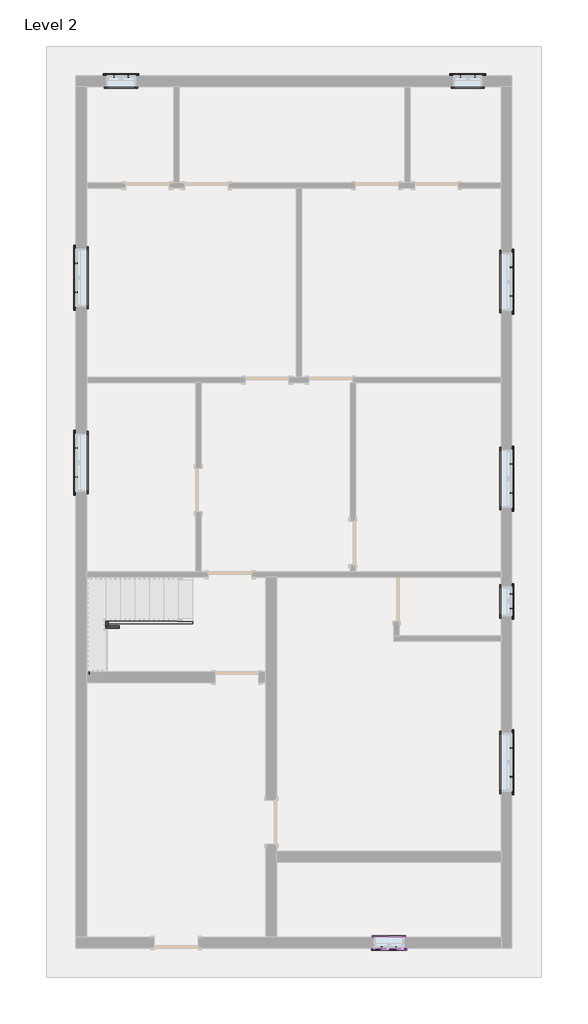
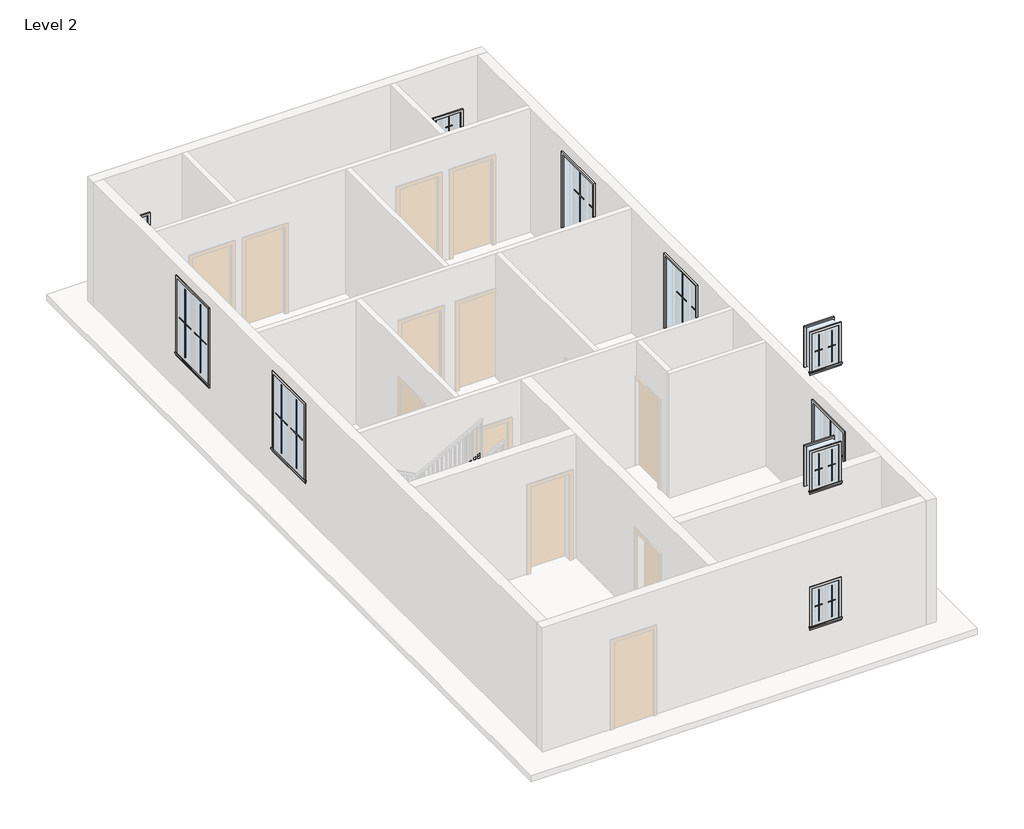
# One storey, part 3 of 3: 44 proxies, 6 members.
"""IFC4 building model written with IfcOpenShell, lengths in millimetres."""

from ifc_helpers import new_model, si_unit, frame, origin, place, context, project, spatial, polyline, outline, extrude, transform, mapped, element, save
from components import muntin_pattern_2x2_muntin_pattern_2x2_2b4d9f72, muntin_pattern_2x2_muntin_pattern_2x2_ef995ed3, muntin_pattern_2x2_muntin_pattern_2x2_53152e2c, muntin_pattern_2x2_muntin_pattern_2x2_e8f3e573, trim_window_exterior_flat_with_sill_b7e4d11c, trim_window_exterior_flat_with_sill_a665a915, trim_window_interior_flat_picture_frame_936b8d2a, trim_window_interior_flat_picture_frame_d485c387

model = new_model("IFC4")

# Units and contexts
model_context = context("Model", 3, world=origin())
ifc_project = project(units=[si_unit("LENGTHUNIT", "METRE", prefix="MILLI")], contexts=[model_context])

# Site, building, storey
site = spatial("IfcSite", under=ifc_project)
building = spatial("IfcBuilding", under=site)
storey = spatial("IfcBuildingStorey", under=building, Name="Level 2", Elevation=3048.0)

# Proxies
placement = place(None, origin())
muntin_pattern_2x2_muntin_pattern_2x2_shape = muntin_pattern_2x2_muntin_pattern_2x2_2b4d9f72(model_context)
element("IfcBuildingElementProxy", 1, Name="Muntin Pattern_2x2 : Muntin Pattern_2x2", ObjectType="Muntin Pattern_2x2 : Muntin Pattern_2x2", at=placement, inside=storey, context=model_context, shape_type="MappedRepresentation", body=[
    mapped(muntin_pattern_2x2_muntin_pattern_2x2_shape, transform((1279.525, 5811.8375, 4032.25), x_axis=(0.0, 1.0, 0.0), y_axis=(-1.0, 0.0, 0.0), z_axis=(0.0, 0.0, 1.0))),
])
element("IfcBuildingElementProxy", 2, Name="Muntin Pattern_2x2 : Muntin Pattern_2x2", ObjectType="Muntin Pattern_2x2 : Muntin Pattern_2x2", at=placement, inside=storey, context=model_context, shape_type="MappedRepresentation", body=[
    mapped(muntin_pattern_2x2_muntin_pattern_2x2_shape, transform((1279.525, 9685.3375, 4032.25), x_axis=(0.0, 1.0, 0.0), y_axis=(-1.0, 0.0, 0.0), z_axis=(0.0, 0.0, 1.0))),
])
element("IfcBuildingElementProxy", 3, Name="Muntin Pattern_2x2 : Muntin Pattern_2x2", ObjectType="Muntin Pattern_2x2 : Muntin Pattern_2x2", at=placement, inside=storey, context=model_context, shape_type="MappedRepresentation", body=[
    mapped(muntin_pattern_2x2_muntin_pattern_2x2_shape, transform((10404.475, 10209.2125, 4032.25), x_axis=(0.0, -1.0, 0.0), y_axis=(1.0, 0.0, 0.0), z_axis=(0.0, 0.0, 1.0))),
])
element("IfcBuildingElementProxy", 4, Name="Muntin Pattern_2x2 : Muntin Pattern_2x2", ObjectType="Muntin Pattern_2x2 : Muntin Pattern_2x2", at=placement, inside=storey, context=model_context, shape_type="MappedRepresentation", body=[
    mapped(muntin_pattern_2x2_muntin_pattern_2x2_shape, transform((10404.475, 6081.7125, 4032.25), x_axis=(0.0, -1.0, 0.0), y_axis=(1.0, 0.0, 0.0), z_axis=(0.0, 0.0, 1.0))),
])
element("IfcBuildingElementProxy", 5, Name="Muntin Pattern_2x2 : Muntin Pattern_2x2", ObjectType="Muntin Pattern_2x2 : Muntin Pattern_2x2", at=placement, inside=storey, context=model_context, shape_type="MappedRepresentation", body=[
    mapped(muntin_pattern_2x2_muntin_pattern_2x2_shape, transform((10404.475, 138.1125, 4032.25), x_axis=(0.0, -1.0, 0.0), y_axis=(1.0, 0.0, 0.0), z_axis=(0.0, 0.0, 1.0))),
])
muntin_pattern_2x2_muntin_pattern_2x2_2_shape = muntin_pattern_2x2_muntin_pattern_2x2_ef995ed3(model_context)
element("IfcBuildingElementProxy", 6, Name="Muntin Pattern_2x2 : Muntin Pattern_2x2", ObjectType="Muntin Pattern_2x2 : Muntin Pattern_2x2", at=placement, inside=storey, context=model_context, shape_type="MappedRepresentation", body=[
    mapped(muntin_pattern_2x2_muntin_pattern_2x2_2_shape, transform((1279.525, 6418.2625, 4032.25), x_axis=(0.0, -1.0, 0.0), y_axis=(1.0, 0.0, 0.0), z_axis=(0.0, 0.0, 1.0))),
])
element("IfcBuildingElementProxy", 7, Name="Muntin Pattern_2x2 : Muntin Pattern_2x2", ObjectType="Muntin Pattern_2x2 : Muntin Pattern_2x2", at=placement, inside=storey, context=model_context, shape_type="MappedRepresentation", body=[
    mapped(muntin_pattern_2x2_muntin_pattern_2x2_2_shape, transform((1279.525, 10291.7625, 4032.25), x_axis=(0.0, -1.0, 0.0), y_axis=(1.0, 0.0, 0.0), z_axis=(0.0, 0.0, 1.0))),
])
element("IfcBuildingElementProxy", 8, Name="Muntin Pattern_2x2 : Muntin Pattern_2x2", ObjectType="Muntin Pattern_2x2 : Muntin Pattern_2x2", at=placement, inside=storey, context=model_context, shape_type="MappedRepresentation", body=[
    mapped(muntin_pattern_2x2_muntin_pattern_2x2_2_shape, transform((10404.475, 9602.7875, 4032.25), x_axis=(0.0, 1.0, 0.0), y_axis=(-1.0, 0.0, 0.0), z_axis=(0.0, 0.0, 1.0))),
])
element("IfcBuildingElementProxy", 9, Name="Muntin Pattern_2x2 : Muntin Pattern_2x2", ObjectType="Muntin Pattern_2x2 : Muntin Pattern_2x2", at=placement, inside=storey, context=model_context, shape_type="MappedRepresentation", body=[
    mapped(muntin_pattern_2x2_muntin_pattern_2x2_2_shape, transform((10404.475, 5475.2875, 4032.25), x_axis=(0.0, 1.0, 0.0), y_axis=(-1.0, 0.0, 0.0), z_axis=(0.0, 0.0, 1.0))),
])
element("IfcBuildingElementProxy", 10, Name="Muntin Pattern_2x2 : Muntin Pattern_2x2", ObjectType="Muntin Pattern_2x2 : Muntin Pattern_2x2", at=placement, inside=storey, context=model_context, shape_type="MappedRepresentation", body=[
    mapped(muntin_pattern_2x2_muntin_pattern_2x2_2_shape, transform((10404.475, -468.3125, 4032.25), x_axis=(0.0, 1.0, 0.0), y_axis=(-1.0, 0.0, 0.0), z_axis=(0.0, 0.0, 1.0))),
])
muntin_pattern_2x2_muntin_pattern_2x2_3_shape = muntin_pattern_2x2_muntin_pattern_2x2_53152e2c(model_context)
element("IfcBuildingElementProxy", 11, Name="Muntin Pattern_2x2 : Muntin Pattern_2x2", ObjectType="Muntin Pattern_2x2 : Muntin Pattern_2x2", at=placement, inside=storey, context=model_context, shape_type="MappedRepresentation", body=[
    mapped(muntin_pattern_2x2_muntin_pattern_2x2_3_shape, transform((10404.475, 3357.5625, 4032.25), x_axis=(0.0, -1.0, 0.0), y_axis=(1.0, 0.0, 0.0), z_axis=(0.0, 0.0, 1.0))),
])
element("IfcBuildingElementProxy", 12, Name="Muntin Pattern_2x2 : Muntin Pattern_2x2", ObjectType="Muntin Pattern_2x2 : Muntin Pattern_2x2", at=placement, inside=storey, context=model_context, shape_type="MappedRepresentation", body=[
    mapped(muntin_pattern_2x2_muntin_pattern_2x2_3_shape, transform((9336.0875, 14214.475, 4032.25), x_axis=(1.0, 0.0, 0.0), y_axis=(0.0, 1.0, 0.0), z_axis=(0.0, 0.0, 1.0))),
])
element("IfcBuildingElementProxy", 13, Name="Muntin Pattern_2x2 : Muntin Pattern_2x2", ObjectType="Muntin Pattern_2x2 : Muntin Pattern_2x2", at=placement, inside=storey, context=model_context, shape_type="MappedRepresentation", body=[
    mapped(muntin_pattern_2x2_muntin_pattern_2x2_3_shape, transform((2071.6875, 14214.475, 4032.25), x_axis=(1.0, 0.0, 0.0), y_axis=(0.0, 1.0, 0.0), z_axis=(0.0, 0.0, 1.0))),
])
element("IfcBuildingElementProxy", 14, Name="Muntin Pattern_2x2 : Muntin Pattern_2x2", ObjectType="Muntin Pattern_2x2 : Muntin Pattern_2x2", at=placement, inside=storey, context=model_context, shape_type="MappedRepresentation", body=[
    mapped(muntin_pattern_2x2_muntin_pattern_2x2_3_shape, transform((7986.7125, -4054.475, 4032.25), x_axis=(-1.0, 0.0, 0.0), y_axis=(0.0, -1.0, 0.0), z_axis=(0.0, 0.0, 1.0))),
])
element("IfcBuildingElementProxy", 15, Name="Muntin Pattern_2x2 : Muntin Pattern_2x2", ObjectType="Muntin Pattern_2x2 : Muntin Pattern_2x2", at=placement, inside=storey, context=model_context, shape_type="MappedRepresentation", body=[
    mapped(muntin_pattern_2x2_muntin_pattern_2x2_3_shape, transform((7986.7125, -4054.475, 7370.6757161), x_axis=(-1.0, 0.0, 0.0), y_axis=(0.0, -1.0, 0.0), z_axis=(0.0, 0.0, 1.0))),
])
element("IfcBuildingElementProxy", 16, Name="Muntin Pattern_2x2 : Muntin Pattern_2x2", ObjectType="Muntin Pattern_2x2 : Muntin Pattern_2x2", at=placement, inside=storey, context=model_context, shape_type="MappedRepresentation", body=[
    mapped(muntin_pattern_2x2_muntin_pattern_2x2_3_shape, transform((7986.7125, -4054.475, 10294.9373604), x_axis=(-1.0, 0.0, 0.0), y_axis=(0.0, -1.0, 0.0), z_axis=(0.0, 0.0, 1.0))),
])
muntin_pattern_2x2_muntin_pattern_2x2_4_shape = muntin_pattern_2x2_muntin_pattern_2x2_e8f3e573(model_context)
element("IfcBuildingElementProxy", 17, Name="Muntin Pattern_2x2 : Muntin Pattern_2x2", ObjectType="Muntin Pattern_2x2 : Muntin Pattern_2x2", at=placement, inside=storey, context=model_context, shape_type="MappedRepresentation", body=[
    mapped(muntin_pattern_2x2_muntin_pattern_2x2_4_shape, transform((10404.475, 3055.9375, 4032.25), x_axis=(0.0, 1.0, 0.0), y_axis=(-1.0, 0.0, 0.0), z_axis=(0.0, 0.0, 1.0))),
])
element("IfcBuildingElementProxy", 18, Name="Muntin Pattern_2x2 : Muntin Pattern_2x2", ObjectType="Muntin Pattern_2x2 : Muntin Pattern_2x2", at=placement, inside=storey, context=model_context, shape_type="MappedRepresentation", body=[
    mapped(muntin_pattern_2x2_muntin_pattern_2x2_4_shape, transform((9637.7125, 14214.475, 4032.25), x_axis=(-1.0, 0.0, 0.0), y_axis=(0.0, -1.0, 0.0), z_axis=(0.0, 0.0, 1.0))),
])
element("IfcBuildingElementProxy", 19, Name="Muntin Pattern_2x2 : Muntin Pattern_2x2", ObjectType="Muntin Pattern_2x2 : Muntin Pattern_2x2", at=placement, inside=storey, context=model_context, shape_type="MappedRepresentation", body=[
    mapped(muntin_pattern_2x2_muntin_pattern_2x2_4_shape, transform((2373.3125, 14214.475, 4032.25), x_axis=(-1.0, 0.0, 0.0), y_axis=(0.0, -1.0, 0.0), z_axis=(0.0, 0.0, 1.0))),
])
element("IfcBuildingElementProxy", 20, Name="Muntin Pattern_2x2 : Muntin Pattern_2x2", ObjectType="Muntin Pattern_2x2 : Muntin Pattern_2x2", at=placement, inside=storey, context=model_context, shape_type="MappedRepresentation", body=[
    mapped(muntin_pattern_2x2_muntin_pattern_2x2_4_shape, transform((7685.0875, -4054.475, 4032.25), x_axis=(1.0, 0.0, 0.0), y_axis=(0.0, 1.0, 0.0), z_axis=(0.0, 0.0, 1.0))),
])
element("IfcBuildingElementProxy", 21, Name="Muntin Pattern_2x2 : Muntin Pattern_2x2", ObjectType="Muntin Pattern_2x2 : Muntin Pattern_2x2", at=placement, inside=storey, context=model_context, shape_type="MappedRepresentation", body=[
    mapped(muntin_pattern_2x2_muntin_pattern_2x2_4_shape, transform((7685.0875, -4054.475, 7370.6757161), x_axis=(1.0, 0.0, 0.0), y_axis=(0.0, 1.0, 0.0), z_axis=(0.0, 0.0, 1.0))),
])
element("IfcBuildingElementProxy", 22, Name="Muntin Pattern_2x2 : Muntin Pattern_2x2", ObjectType="Muntin Pattern_2x2 : Muntin Pattern_2x2", at=placement, inside=storey, context=model_context, shape_type="MappedRepresentation", body=[
    mapped(muntin_pattern_2x2_muntin_pattern_2x2_4_shape, transform((7685.0875, -4054.475, 10294.9373604), x_axis=(1.0, 0.0, 0.0), y_axis=(0.0, 1.0, 0.0), z_axis=(0.0, 0.0, 1.0))),
])
trim_window_exterior_flat_with_sill_shape = trim_window_exterior_flat_with_sill_b7e4d11c(model_context)
element("IfcBuildingElementProxy", 23, Name="Trim-Window-Exterior-Flat : with Sill", ObjectType="Trim-Window-Exterior-Flat : with Sill", at=placement, inside=storey, context=model_context, shape_type="MappedRepresentation", body=[
    mapped(trim_window_exterior_flat_with_sill_shape, transform((1270.0, 6115.05, 5791.2), x_axis=(0.0, -1.0, 0.0), y_axis=(0.0, 0.0, 1.0), z_axis=(-1.0, 0.0, 0.0))),
])
element("IfcBuildingElementProxy", 24, Name="Trim-Window-Exterior-Flat : with Sill", ObjectType="Trim-Window-Exterior-Flat : with Sill", at=placement, inside=storey, context=model_context, shape_type="MappedRepresentation", body=[
    mapped(trim_window_exterior_flat_with_sill_shape, transform((1270.0, 9988.55, 5791.2), x_axis=(0.0, -1.0, 0.0), y_axis=(0.0, 0.0, 1.0), z_axis=(-1.0, 0.0, 0.0))),
])
element("IfcBuildingElementProxy", 25, Name="Trim-Window-Exterior-Flat : with Sill", ObjectType="Trim-Window-Exterior-Flat : with Sill", at=placement, inside=storey, context=model_context, shape_type="MappedRepresentation", body=[
    mapped(trim_window_exterior_flat_with_sill_shape, transform((10414.0, 9906.0, 5791.2), x_axis=(0.0, 1.0, 0.0), y_axis=(0.0, 0.0, 1.0), z_axis=(1.0, 0.0, 0.0))),
])
element("IfcBuildingElementProxy", 26, Name="Trim-Window-Exterior-Flat : with Sill", ObjectType="Trim-Window-Exterior-Flat : with Sill", at=placement, inside=storey, context=model_context, shape_type="MappedRepresentation", body=[
    mapped(trim_window_exterior_flat_with_sill_shape, transform((10414.0, 5778.5, 5791.2), x_axis=(0.0, 1.0, 0.0), y_axis=(0.0, 0.0, 1.0), z_axis=(1.0, 0.0, 0.0))),
])
element("IfcBuildingElementProxy", 27, Name="Trim-Window-Exterior-Flat : with Sill", ObjectType="Trim-Window-Exterior-Flat : with Sill", at=placement, inside=storey, context=model_context, shape_type="MappedRepresentation", body=[
    mapped(trim_window_exterior_flat_with_sill_shape, transform((10414.0, -165.1, 5791.2), x_axis=(0.0, 1.0, 0.0), y_axis=(0.0, 0.0, 1.0), z_axis=(1.0, 0.0, 0.0))),
])
trim_window_exterior_flat_with_sill_2_shape = trim_window_exterior_flat_with_sill_a665a915(model_context)
element("IfcBuildingElementProxy", 28, Name="Trim-Window-Exterior-Flat : with Sill", ObjectType="Trim-Window-Exterior-Flat : with Sill", at=placement, inside=storey, context=model_context, shape_type="MappedRepresentation", body=[
    mapped(trim_window_exterior_flat_with_sill_2_shape, transform((10414.0, 3206.75, 4876.8), x_axis=(0.0, 1.0, 0.0), y_axis=(0.0, 0.0, 1.0), z_axis=(1.0, 0.0, 0.0))),
])
element("IfcBuildingElementProxy", 29, Name="Trim-Window-Exterior-Flat : with Sill", ObjectType="Trim-Window-Exterior-Flat : with Sill", at=placement, inside=storey, context=model_context, shape_type="MappedRepresentation", body=[
    mapped(trim_window_exterior_flat_with_sill_2_shape, transform((9486.9, 14224.0, 4876.8), x_axis=(-1.0, 0.0, 0.0), y_axis=(0.0, 0.0, 1.0), z_axis=(0.0, 1.0, 0.0))),
])
element("IfcBuildingElementProxy", 30, Name="Trim-Window-Exterior-Flat : with Sill", ObjectType="Trim-Window-Exterior-Flat : with Sill", at=placement, inside=storey, context=model_context, shape_type="MappedRepresentation", body=[
    mapped(trim_window_exterior_flat_with_sill_2_shape, transform((2222.5, 14224.0, 4876.8), x_axis=(-1.0, 0.0, 0.0), y_axis=(0.0, 0.0, 1.0), z_axis=(0.0, 1.0, 0.0))),
])
element("IfcBuildingElementProxy", 31, Name="Trim-Window-Exterior-Flat : with Sill", ObjectType="Trim-Window-Exterior-Flat : with Sill", at=placement, inside=storey, context=model_context, shape_type="MappedRepresentation", body=[
    mapped(trim_window_exterior_flat_with_sill_2_shape, transform((7835.9, -4064.0, 4876.8), x_axis=(1.0, 0.0, 0.0), y_axis=(0.0, 0.0, 1.0), z_axis=(0.0, -1.0, 0.0))),
])
element("IfcBuildingElementProxy", 32, Name="Trim-Window-Exterior-Flat : with Sill", ObjectType="Trim-Window-Exterior-Flat : with Sill", at=placement, inside=storey, context=model_context, shape_type="MappedRepresentation", body=[
    mapped(trim_window_exterior_flat_with_sill_2_shape, transform((7835.9, -4064.0, 8215.2257161), x_axis=(1.0, 0.0, 0.0), y_axis=(0.0, 0.0, 1.0), z_axis=(0.0, -1.0, 0.0))),
])
element("IfcBuildingElementProxy", 33, Name="Trim-Window-Exterior-Flat : with Sill", ObjectType="Trim-Window-Exterior-Flat : with Sill", at=placement, inside=storey, context=model_context, shape_type="MappedRepresentation", body=[
    mapped(trim_window_exterior_flat_with_sill_2_shape, transform((7835.9, -4064.0, 11139.4873604), x_axis=(1.0, 0.0, 0.0), y_axis=(0.0, 0.0, 1.0), z_axis=(0.0, -1.0, 0.0))),
])
trim_window_interior_flat_picture_frame_shape = trim_window_interior_flat_picture_frame_936b8d2a(model_context)
element("IfcBuildingElementProxy", 34, Name="Trim-Window-Interior-Flat : Picture Frame", ObjectType="Trim-Window-Interior-Flat : Picture Frame", at=placement, inside=storey, context=model_context, shape_type="MappedRepresentation", body=[
    mapped(trim_window_interior_flat_picture_frame_shape, transform((1498.6, 6115.05, 5791.2), x_axis=(0.0, 1.0, 0.0), y_axis=(0.0, 0.0, 1.0), z_axis=(1.0, 0.0, 0.0))),
])
element("IfcBuildingElementProxy", 35, Name="Trim-Window-Interior-Flat : Picture Frame", ObjectType="Trim-Window-Interior-Flat : Picture Frame", at=placement, inside=storey, context=model_context, shape_type="MappedRepresentation", body=[
    mapped(trim_window_interior_flat_picture_frame_shape, transform((1498.6, 9988.55, 5791.2), x_axis=(0.0, 1.0, 0.0), y_axis=(0.0, 0.0, 1.0), z_axis=(1.0, 0.0, 0.0))),
])
element("IfcBuildingElementProxy", 36, Name="Trim-Window-Interior-Flat : Picture Frame", ObjectType="Trim-Window-Interior-Flat : Picture Frame", at=placement, inside=storey, context=model_context, shape_type="MappedRepresentation", body=[
    mapped(trim_window_interior_flat_picture_frame_shape, transform((10185.4, 9906.0, 5791.2), x_axis=(0.0, -1.0, 0.0), y_axis=(0.0, 0.0, 1.0), z_axis=(-1.0, 0.0, 0.0))),
])
element("IfcBuildingElementProxy", 37, Name="Trim-Window-Interior-Flat : Picture Frame", ObjectType="Trim-Window-Interior-Flat : Picture Frame", at=placement, inside=storey, context=model_context, shape_type="MappedRepresentation", body=[
    mapped(trim_window_interior_flat_picture_frame_shape, transform((10185.4, 5778.5, 5791.2), x_axis=(0.0, -1.0, 0.0), y_axis=(0.0, 0.0, 1.0), z_axis=(-1.0, 0.0, 0.0))),
])
element("IfcBuildingElementProxy", 38, Name="Trim-Window-Interior-Flat : Picture Frame", ObjectType="Trim-Window-Interior-Flat : Picture Frame", at=placement, inside=storey, context=model_context, shape_type="MappedRepresentation", body=[
    mapped(trim_window_interior_flat_picture_frame_shape, transform((10185.4, -165.1, 5791.2), x_axis=(0.0, -1.0, 0.0), y_axis=(0.0, 0.0, 1.0), z_axis=(-1.0, 0.0, 0.0))),
])
trim_window_interior_flat_picture_frame_2_shape = trim_window_interior_flat_picture_frame_d485c387(model_context)
element("IfcBuildingElementProxy", 39, Name="Trim-Window-Interior-Flat : Picture Frame", ObjectType="Trim-Window-Interior-Flat : Picture Frame", at=placement, inside=storey, context=model_context, shape_type="MappedRepresentation", body=[
    mapped(trim_window_interior_flat_picture_frame_2_shape, transform((10185.4, 3206.75, 4876.8), x_axis=(0.0, -1.0, 0.0), y_axis=(0.0, 0.0, 1.0), z_axis=(-1.0, 0.0, 0.0))),
])
element("IfcBuildingElementProxy", 40, Name="Trim-Window-Interior-Flat : Picture Frame", ObjectType="Trim-Window-Interior-Flat : Picture Frame", at=placement, inside=storey, context=model_context, shape_type="MappedRepresentation", body=[
    mapped(trim_window_interior_flat_picture_frame_2_shape, transform((9486.9, 13995.4, 4876.8), x_axis=(1.0, 0.0, 0.0), y_axis=(0.0, 0.0, 1.0), z_axis=(0.0, -1.0, 0.0))),
])
element("IfcBuildingElementProxy", 41, Name="Trim-Window-Interior-Flat : Picture Frame", ObjectType="Trim-Window-Interior-Flat : Picture Frame", at=placement, inside=storey, context=model_context, shape_type="MappedRepresentation", body=[
    mapped(trim_window_interior_flat_picture_frame_2_shape, transform((2222.5, 13995.4, 4876.8), x_axis=(1.0, 0.0, 0.0), y_axis=(0.0, 0.0, 1.0), z_axis=(0.0, -1.0, 0.0))),
])
element("IfcBuildingElementProxy", 42, Name="Trim-Window-Interior-Flat : Picture Frame", ObjectType="Trim-Window-Interior-Flat : Picture Frame", at=placement, inside=storey, context=model_context, shape_type="MappedRepresentation", body=[
    mapped(trim_window_interior_flat_picture_frame_2_shape, transform((7835.9, -3835.4, 4876.8), x_axis=(-1.0, 0.0, 0.0), y_axis=(0.0, 0.0, 1.0), z_axis=(0.0, 1.0, 0.0))),
])
element("IfcBuildingElementProxy", 43, Name="Trim-Window-Interior-Flat : Picture Frame", ObjectType="Trim-Window-Interior-Flat : Picture Frame", at=placement, inside=storey, context=model_context, shape_type="MappedRepresentation", body=[
    mapped(trim_window_interior_flat_picture_frame_2_shape, transform((7835.9, -3835.4, 8215.2257161), x_axis=(-1.0, 0.0, 0.0), y_axis=(0.0, 0.0, 1.0), z_axis=(0.0, 1.0, 0.0))),
])
element("IfcBuildingElementProxy", 44, Name="Trim-Window-Interior-Flat : Picture Frame", ObjectType="Trim-Window-Interior-Flat : Picture Frame", at=placement, inside=storey, context=model_context, shape_type="MappedRepresentation", body=[
    mapped(trim_window_interior_flat_picture_frame_2_shape, transform((7835.9, -3835.4, 11139.4873604), x_axis=(-1.0, 0.0, 0.0), y_axis=(0.0, 0.0, 1.0), z_axis=(0.0, 1.0, 0.0))),
])

# Members
element("IfcMember", 45, ObjectType="Stringer - 2\" Width", at=placement, inside=storey, context=model_context, shape_type="SweptSolid", body=[
    extrude(outline(polyline([(3048.0, 3727.9146873), (3255.5983948, 3727.9146873), (4243.3761726, 1949.9146873), (3894.6974984, 1949.9146873), (3048.0, 3473.9701845), (3048.0, 3727.9146873)])), frame((0.0, 2743.2, 0.0), z_axis=(0.0, 1.0, 0.0), x_axis=(0.0, 0.0, 1.0)), (0.0, 0.0, 1.0), 50.8),
])
element("IfcMember", 46, ObjectType="Stringer - 2\" Width", at=placement, inside=storey, context=model_context, shape_type="SweptSolid", body=[
    extrude(outline(polyline([(1899.1146873, 2794.0), (1949.9146873, 2794.0), (1949.9146873, 2692.4), (1899.1146873, 2692.4), (1899.1146873, 2794.0)])), frame((0.0, 0.0, 4004.7333333), z_axis=(0.0, 0.0, 1.0), x_axis=(1.0, 0.0, 0.0)), (0.0, 0.0, 1.0), 304.8),
])
element("IfcMember", 47, ObjectType="Stringer - 2\" Width", at=placement, inside=storey, context=model_context, shape_type="SweptSolid", body=[
    extrude(outline(polyline([(4440.9317281, 1899.1146873), (4092.253054, 1899.1146873), (5108.253054, 3727.9146873), (5456.9317281, 3727.9146873), (4440.9317281, 1899.1146873)])), frame((0.0, 2641.6, 0.0), z_axis=(0.0, 1.0, 0.0), x_axis=(0.0, 0.0, 1.0)), (0.0, 0.0, 1.0), 50.8),
])
element("IfcMember", 48, ObjectType="Stringer - 2\" Width", at=placement, inside=storey, context=model_context, shape_type="SweptSolid", body=[
    extrude(outline(polyline([(3048.0, 3727.9146873), (3255.5983948, 3727.9146873), (4309.5333333, 1830.8317979), (4309.5333333, 1498.6), (4145.4278803, 1498.6), (3048.0, 3473.9701845), (3048.0, 3727.9146873)])), frame((0.0, 3708.4, 0.0), z_axis=(0.0, 1.0, 0.0), x_axis=(0.0, 0.0, 1.0)), (0.0, 0.0, 1.0), 50.8),
])
element("IfcMember", 49, ObjectType="Stringer - 2\" Width", at=placement, inside=storey, context=model_context, shape_type="SweptSolid", body=[
    extrude(outline(polyline([(1447.8, 3759.2), (1498.6, 3759.2), (1498.6, 1727.2), (1447.8, 1727.2), (1447.8, 3759.2)])), frame((0.0, 0.0, 4004.7333333), z_axis=(0.0, 0.0, 1.0), x_axis=(1.0, 0.0, 0.0)), (0.0, 0.0, 1.0), 304.8),
])
element("IfcMember", 50, ObjectType="Stringer - 2\" Width", at=placement, inside=storey, context=model_context, shape_type="SweptSolid", body=[
    extrude(outline(polyline([(4190.2013463, 1447.8), (4004.7333333, 1447.8), (4004.7333333, 1741.5791901), (5108.253054, 3727.9146873), (5456.9317281, 3727.9146873), (4190.2013463, 1447.8)])), frame((0.0, 1676.4, 0.0), z_axis=(0.0, 1.0, 0.0), x_axis=(0.0, 0.0, 1.0)), (0.0, 0.0, 1.0), 50.8),
])

save(model, "model.ifc")

# Revit data of these elements
# Type "Muntin Pattern_2x2 : Muntin Pattern_2x2"
#   Width [instance default] = 4' - 0"
#   Thickness = 0' - 0 1/2"
#   Height [instance default] = 4' - 0"
#   Distance = 0' - 0 3/4"
#   Interior Material [instance default] = none
#   Exterior Material [instance default] = none
#   Default Elevation = 0
# Type "Trim-Window-Exterior-Flat : with Sill"
#   Trim Width = 0' - 2 1/4"
#   Trim Thickness_Picture Frame = 0' - 1 1/4"
#   Trim Thickness_with Sill = 0' - 0 3/4"
#   Sill Thickness = 0' - 1 1/4"
#   Opening Width [instance default] = 2' - 0"
#   Opening Height [instance default] = 3' - 0"
#   Default Elevation = 4' - 0"
#   Sill = yes
#   Picture Frame = no
#   Trim Material [instance default] = none
# Type "Trim-Window-Interior-Flat : Picture Frame"
#   Trim Thickness_Picture Frame = 0' - 1 1/4"
#   Trim Width = 0' - 2 1/4"
#   Trim Thickness_with Sill = 0' - 0 3/4"
#   Sill Thickness = 0' - 1 1/4"
#   Opening Width [instance default] = 2' - 0"
#   Opening Height [instance default] = 3' - 0"
#   Default Elevation = 4' - 0"
#   Sill = no
#   Picture Frame = yes
#   Trim Material [instance default] = none
# Elements 1, 2, 3, 4, 5, 6, 7, 8, 9, 10 (IfcBuildingElementProxy, "Muntin Pattern_2x2 : Muntin Pattern_2x2")
#   Width = 1' - 6 5/8"
#   Height = 5' - 6 1/2"
#   Interior Material = Wood - Stained
#   Exterior Material = Clad - White
#   Phase Created = New Construction
#   Materials on its faces: "Clad - White", "Wood - Stained"
# Elements 11, 12, 13, 14, 15, 16, 17, 18, 19, 20, 21, 22 (IfcBuildingElementProxy, "Muntin Pattern_2x2 : Muntin Pattern_2x2")
#   Width = 0' - 6 5/8"
#   Height = 2' - 6 1/2"
#   Interior Material = Wood - Stained
#   Exterior Material = Clad - White
#   Phase Created = New Construction
#   Materials on its faces: "Clad - White", "Wood - Stained"
# Elements 23, 24, 25, 26, 27 (IfcBuildingElementProxy, "Trim-Window-Exterior-Flat : with Sill")
#   Opening Width = 4' - 0"
#   Opening Height = 6' - 0"
#   Trim Material = Clad - White
#   Phase Created = New Construction
#   Materials on its faces: "Clad - White"
# Elements 28, 29, 30, 31, 32, 33 (IfcBuildingElementProxy, "Trim-Window-Exterior-Flat : with Sill")
#   Opening Width = 2' - 0"
#   Opening Height = 3' - 0"
#   Trim Material = Clad - White
#   Phase Created = New Construction
#   Materials on its faces: "Clad - White"
# Elements 34, 35, 36, 37, 38 (IfcBuildingElementProxy, "Trim-Window-Interior-Flat : Picture Frame")
#   Opening Width = 4' - 0"
#   Opening Height = 6' - 0"
#   Trim Material = Wood - Stained
#   Phase Created = New Construction
#   Materials on its faces: "Wood - Stained"
# Elements 39, 40, 41, 42, 43, 44 (IfcBuildingElementProxy, "Trim-Window-Interior-Flat : Picture Frame")
#   Opening Width = 2' - 0"
#   Opening Height = 3' - 0"
#   Trim Material = Wood - Stained
#   Phase Created = New Construction
#   Materials on its faces: "Wood - Stained"
# Elements 45, 46, 47, 48, 49, 50 (IfcMember, "Stringer - 2\" Width")
#   Phase Created = New Construction
# Materials
#   "Clad - White": class "Wood", colour RGB 242 242 238, transparency 0, Cost = 0
#   "Wood - Stained": class "Wood", colour RGB 224 178 126, transparency 0, Cost = 0
